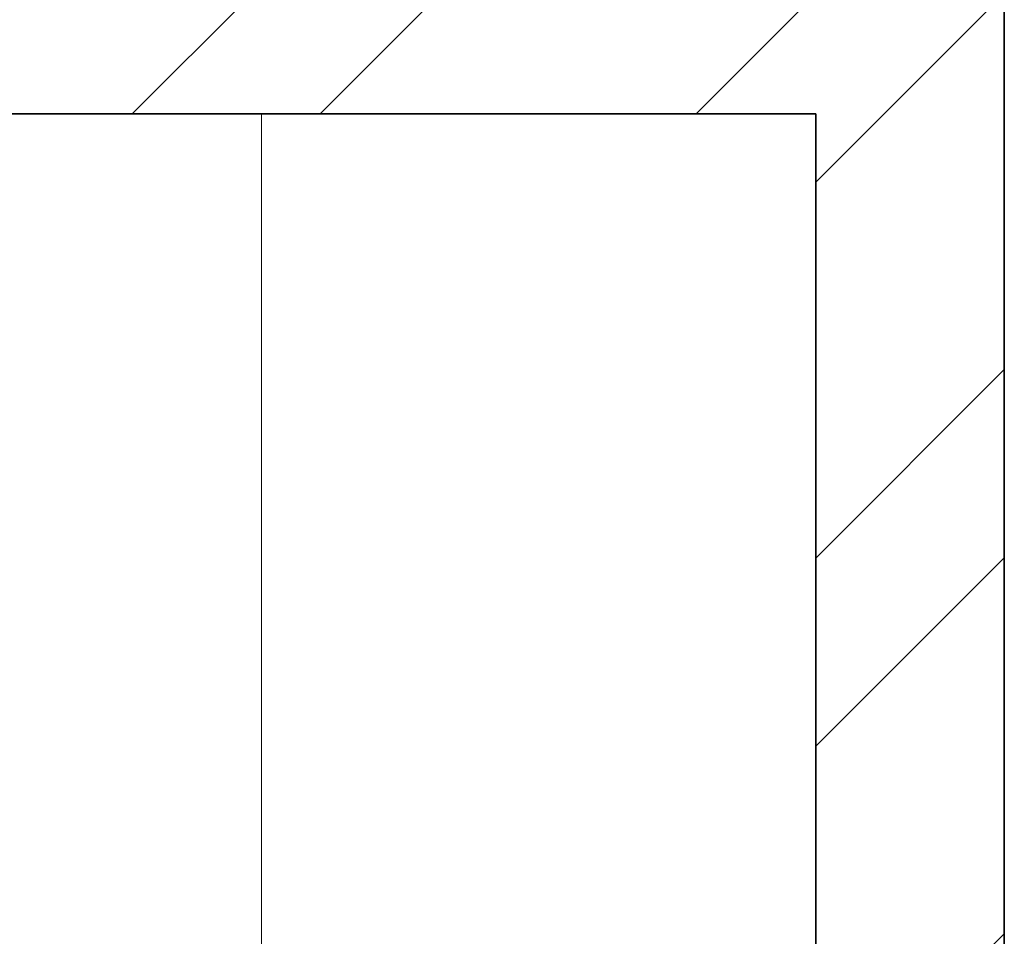
# Model space of a CAD drawing. Units: inches. Extents: x 1885 to 2748, y 783 to 2421.
# Tile 115 of 117: x 2595 to 2618, y 2093 to 2115. Entities that reach past the tile are written whole.
import ezdxf

# ---------------------------------------------------------------- set-up
doc = ezdxf.new("R2010")
doc.units = ezdxf.units.IN
doc.layers.add('A-FLOR-CASE', color=9, linetype='Continuous', lineweight=18)
doc.layers.add('A-WALL', color=7, linetype='Continuous', lineweight=35)
doc.layers.add('A-WALL-PATT', color=85, linetype='Continuous', lineweight=13, true_color=0x58ba48)

msp = doc.modelspace()

# ---------------------------------------------------------------- hatches: boundary and pattern name
at = {"layer": 'A-WALL-PATT'}
h = msp.add_hatch(dxfattribs=at)
h.set_pattern_fill('ANSI32', color=256)
h.paths.add_polyline_path([(2007.772, 2318.006), (1980.774, 2318.006), (1980.774, 2281.215), (1985.274, 2281.215), (1985.274, 2313.506), (2007.772, 2313.506), (2007.772, 2315.756)])
h.paths.add_polyline_path([(2094.324, 2318.006), (2067.772, 2318.006), (2067.772, 2313.506), (2094.324, 2313.506), (2094.324, 2315.756)])
h.paths.add_polyline_path([(2131.367, 2315.756), (2131.367, 2318.006), (2131.189, 2318.006), (2112.609, 2318.006), (2112.609, 2313.506), (2117.274, 2313.506), (2117.274, 2255.201), (2121.774, 2255.201), (2121.774, 2313.506), (2131.367, 2313.506)])
h.paths.add_polyline_path([(2190.512, 2318.006), (2155.367, 2318.006), (2155.367, 2313.506), (2169.774, 2313.506), (2169.774, 2229.506), (2121.774, 2229.506), (2121.774, 2233.451), (2119.524, 2233.451), (2117.274, 2233.451), (2117.274, 2201.101), (2121.774, 2201.101), (2121.774, 2225.006), (2169.774, 2225.006), (2169.774, 2165.006), (2306.274, 2165.006), (2306.274, 2066.006), (2310.774, 2066.006), (2344.274, 2066.006), (2486.274, 2066.006), (2486.274, 1886.006), (2483.02, 1886.006), (2483.02, 1881.506), (2486.274, 1881.506), (2486.274, 1880.678), (2490.774, 1880.678), (2490.774, 2070.506), (2344.274, 2070.506), (2310.774, 2070.506), (2310.774, 2165.006), (2310.774, 2173.636), (2308.524, 2173.636), (2306.274, 2173.636), (2306.274, 2169.506), (2174.274, 2169.506), (2174.274, 2313.506), (2190.512, 2313.506), (2190.512, 2315.756)])
h.paths.add_polyline_path([(1985.274, 2221.215), (1980.774, 2221.215), (1980.774, 2165.006), (1992.774, 2165.006), (1992.774, 2141.927), (1997.274, 2141.927), (1997.274, 2165.006), (2117.274, 2165.006), (2117.274, 2163.126), (2121.774, 2163.126), (2121.774, 2172.734), (2119.524, 2172.734), (2117.274, 2172.734), (2117.274, 2169.506), (1985.274, 2169.506)])
h.paths.add_polyline_path([(1997.274, 2105.927), (1992.774, 2105.927), (1992.774, 2070.506), (2016.774, 2070.506), (2016.774, 2059.123), (2019.024, 2059.123), (2021.274, 2059.123), (2021.274, 2070.506), (2117.274, 2070.506), (2117.274, 2022.506), (2114.423, 2022.506), (2114.423, 2018.006), (2123.627, 2018.006), (2123.627, 2020.256), (2123.627, 2022.506), (2121.774, 2022.506), (2121.774, 2142.587), (2119.524, 2142.587), (2117.274, 2142.587), (2117.274, 2075.006), (1997.274, 2075.006)])
h.paths.add_polyline_path([(2092.029, 2020.256), (2092.029, 2022.506), (2021.274, 2022.506), (2021.274, 2035.123), (2016.774, 2035.123), (2016.774, 2018.006), (2016.774, 1978.784), (2021.274, 1978.784), (2021.274, 2018.006), (2092.029, 2018.006)])
h.paths.add_polyline_path([(2260.938, 2022.506), (2153.105, 2022.506), (2153.105, 2020.256), (2153.105, 2018.006), (2155.274, 2018.006), (2155.274, 1886.006), (2107.629, 1886.006), (2107.629, 1881.506), (2182.911, 1881.506), (2182.911, 1883.756), (2182.911, 1886.006), (2159.774, 1886.006), (2159.774, 2018.006), (2260.938, 2018.006), (2260.938, 2020.256)])
h.paths.add_polyline_path([(2047.629, 1883.756), (2047.629, 1886.006), (2021.274, 1886.006), (2021.274, 1918.784), (2019.024, 1918.784), (2016.774, 1918.784), (2016.774, 1881.506), (2047.629, 1881.506)])
h.paths.add_polyline_path([(2306.361, 1883.756), (2306.361, 1886.006), (2296.274, 1886.006), (2296.274, 1982.006), (2316.535, 1982.006), (2316.535, 1984.256), (2316.535, 1986.506), (2296.274, 1986.506), (2296.274, 2022.506), (2289.276, 2022.506), (2289.276, 2018.006), (2291.774, 2018.006), (2291.774, 1886.006), (2242.911, 1886.006), (2242.911, 1881.506), (2306.361, 1881.506)], flags=17)
h.paths.add_polyline_path([(1985.274, 1843.006), (2021.6, 1843.006), (2021.534, 1845.441), (2021.477, 1847.506), (1980.774, 1847.506), (1980.774, 1809.446), (1985.274, 1809.446)])
h.paths.add_polyline_path([(2131.482, 1845.256), (2131.482, 1847.506), (2081.534, 1847.506), (2081.534, 1843.006), (2117.274, 1843.006), (2117.274, 1784.147), (2119.524, 1784.147), (2121.774, 1784.147), (2121.774, 1843.006), (2131.482, 1843.006)])
h.paths.add_polyline_path([(2203.886, 1847.506), (2155.482, 1847.506), (2155.482, 1843.006), (2169.774, 1843.006), (2169.774, 1759.006), (2121.774, 1759.006), (2121.774, 1761.457), (2117.274, 1761.457), (2117.274, 1730.429), (2121.774, 1730.429), (2121.774, 1754.506), (2177.421, 1754.506), (2177.421, 1756.756), (2177.421, 1759.006), (2174.274, 1759.006), (2174.274, 1843.006), (2203.886, 1843.006)])
h.paths.add_polyline_path([(2335.554, 1845.256), (2335.554, 1847.506), (2239.886, 1847.506), (2239.886, 1843.006), (2306.274, 1843.006), (2306.274, 1759.006), (2199.486, 1759.006), (2199.486, 1754.506), (2310.774, 1754.506), (2310.774, 1843.006), (2335.554, 1843.006)])
h.paths.add_polyline_path([(2348.774, 2022.506), (2344.274, 2022.506), (2344.274, 1986.506), (2341.681, 1986.506), (2341.681, 1982.006), (2344.274, 1982.006), (2344.274, 1886.006), (2330.361, 1886.006), (2330.361, 1881.506), (2361.627, 1881.506), (2361.627, 1883.756), (2361.627, 1886.006), (2348.774, 1886.006)], flags=17)
h.paths.add_polyline_path([(2283.251, 2315.756), (2283.251, 2318.006), (2238.512, 2318.006), (2238.512, 2313.506), (2283.251, 2313.506)], flags=17)
h.paths.add_polyline_path([(2363.274, 2348.006), (2388.677, 2348.006), (2388.677, 2350.256), (2388.677, 2352.506), (2358.774, 2352.506), (2358.774, 2348.006), (2358.774, 2318.006), (2344.481, 2318.006), (2344.481, 2313.506), (2358.774, 2313.506), (2358.774, 2229.506), (2310.774, 2229.506), (2310.774, 2231.952), (2306.274, 2231.952), (2306.274, 2205.611), (2310.774, 2205.611), (2310.774, 2225.006), (2358.774, 2225.006), (2358.774, 2211.506), (2452.329, 2211.506), (2452.329, 2213.756), (2452.329, 2216.006), (2363.274, 2216.006), (2363.274, 2318.006)])
h.paths.add_polyline_path([(2310.774, 2313.506), (2320.481, 2313.506), (2320.481, 2315.756), (2320.481, 2318.006), (2302.728, 2318.006), (2302.728, 2313.506), (2306.274, 2313.506), (2306.274, 2251.076), (2310.774, 2251.076)], flags=17)
h.paths.add_polyline_path([(2490.774, 2352.506), (2486.274, 2352.506), (2448.677, 2352.506), (2448.677, 2348.006), (2486.274, 2348.006), (2486.274, 2318.006), (2486.274, 2216.006), (2481.78, 2216.006), (2481.78, 2211.506), (2486.274, 2211.506), (2486.274, 2165.006), (2493.289, 2165.006), (2493.289, 2167.256), (2493.289, 2169.506), (2490.774, 2169.506), (2490.774, 2313.506), (2494.429, 2313.506), (2494.429, 2318.006), (2490.774, 2318.006)])
h.paths.add_polyline_path([(2534.653, 2318.006), (2515.691, 2318.006), (2515.691, 2313.506), (2534.653, 2313.506), (2534.653, 2315.756)])
h.paths.add_polyline_path([(2618.274, 2318.006), (2594.653, 2318.006), (2594.653, 2313.506), (2613.774, 2313.506), (2613.774, 2281.706), (2618.274, 2281.706)])
h.paths.add_polyline_path([(2618.274, 2221.706), (2613.774, 2221.706), (2613.774, 2169.506), (2554.019, 2169.506), (2554.019, 2165.006), (2613.774, 2165.006), (2613.774, 2152.878), (2618.274, 2152.878)])
h.paths.add_polyline_path([(2618.274, 2128.878), (2616.024, 2128.878), (2613.774, 2128.878), (2613.774, 2117.006), (2529.774, 2117.006), (2529.774, 2165.006), (2532.848, 2165.006), (2532.848, 2169.506), (2522.867, 2169.506), (2522.867, 2165.006), (2525.274, 2165.006), (2525.274, 2117.006), (2525.274, 2112.506), (2525.274, 2108.576), (2529.774, 2108.576), (2529.774, 2112.506), (2613.774, 2112.506), (2613.774, 2080.19), (2618.274, 2080.19)])
h.paths.add_polyline_path([(2618.274, 2044.19), (2616.024, 2044.19), (2613.774, 2044.19), (2613.774, 2015.506), (2529.774, 2015.506), (2529.774, 2088.582), (2527.524, 2088.582), (2525.274, 2088.582), (2525.274, 2011.006), (2613.774, 2011.006), (2613.774, 1956.755), (2618.274, 1956.755)])
h.paths.add_polyline_path([(2618.274, 1881.506), (2618.274, 1896.755), (2613.774, 1896.755), (2613.774, 1881.506), (2613.774, 1847.506), (2592.715, 1847.506), (2592.715, 1843.006), (2613.774, 1843.006), (2613.774, 1765.006), (2613.774, 1760.506), (2609.621, 1760.506), (2609.621, 1756.006), (2613.774, 1756.006), (2613.774, 1660.006), (2608.544, 1660.006), (2608.544, 1655.506), (2613.774, 1655.506), (2613.774, 1508.158), (2618.274, 1508.158)])
h.paths.add_polyline_path([(2565.774, 1843.006), (2568.997, 1843.006), (2568.997, 1847.506), (2490.774, 1847.506), (2490.774, 1849.7), (2488.524, 1849.7), (2486.274, 1849.7), (2486.274, 1847.506), (2477.274, 1847.506), (2477.274, 1838.506), (2477.274, 1821.493), (2486.274, 1821.493), (2486.274, 1838.506), (2561.274, 1838.506), (2561.274, 1765.006), (2486.274, 1765.006), (2486.274, 1786.157), (2477.274, 1786.157), (2477.274, 1765.006), (2477.274, 1756.006), (2486.274, 1756.006), (2565.774, 1756.006), (2585.621, 1756.006), (2585.621, 1758.256), (2585.621, 1760.506), (2565.774, 1760.506), (2565.774, 1765.006)])
h.paths.add_polyline_path([(2486.274, 1651.006), (2561.274, 1651.006), (2561.274, 1567.006), (2486.274, 1567.006), (2486.274, 1591.321), (2477.274, 1591.321), (2477.274, 1567.006), (2477.274, 1558.006), (2477.274, 1555.439), (2481.774, 1555.439), (2481.774, 1558.006), (2568.653, 1558.006), (2568.653, 1560.256), (2568.653, 1562.506), (2565.774, 1562.506), (2565.774, 1655.506), (2584.544, 1655.506), (2584.544, 1657.756), (2584.544, 1660.006), (2565.774, 1660.006), (2486.274, 1660.006), (2477.274, 1660.006), (2477.274, 1651.006), (2477.274, 1632.989), (2486.274, 1632.989)])
h.paths.add_polyline_path([(2449.967, 1883.756), (2449.967, 1886.006), (2421.627, 1886.006), (2421.627, 1881.506), (2449.967, 1881.506)], flags=17)
h.paths.add_polyline_path([(2447.274, 1847.506), (2395.554, 1847.506), (2395.554, 1843.006), (2442.774, 1843.006), (2442.774, 1809.27), (2447.274, 1809.27)])
h.paths.add_polyline_path([(1985.274, 1749.446), (1980.774, 1749.446), (1980.774, 1694.504), (1985.274, 1694.504), (1985.274, 1694.506), (1986.897, 1694.506), (1986.897, 1697.78), (1986.897, 1699.006), (1985.274, 1699.006)])
h.paths.add_polyline_path([(2152.774, 1699.006), (2121.774, 1699.006), (2121.774, 1703.668), (2119.524, 1703.668), (2117.274, 1703.668), (2117.274, 1699.006), (2009.219, 1699.006), (2009.219, 1694.506), (2148.274, 1694.506), (2148.274, 1692.631), (2152.774, 1692.631)])
h.paths.add_polyline_path([(2016.274, 1694.506), (2011.774, 1694.506), (2011.774, 1558.006), (2040.806, 1558.006), (2040.806, 1560.256), (2040.806, 1562.506), (2016.274, 1562.506)])
h.paths.add_polyline_path([(2152.774, 1663.017), (2150.524, 1663.017), (2148.274, 1663.017), (2148.274, 1562.506), (2100.806, 1562.506), (2100.806, 1558.006), (2165.119, 1558.006), (2165.119, 1560.256), (2165.119, 1562.506), (2152.774, 1562.506), (2152.774, 1610.506), (2224.774, 1610.506), (2224.774, 1607.99), (2229.274, 1607.99), (2229.274, 1615.006), (2152.774, 1615.006)])
h.paths.add_polyline_path([(2238.613, 1560.256), (2238.613, 1562.506), (2229.274, 1562.506), (2229.274, 1588.756), (2227.024, 1588.763), (2224.774, 1588.771), (2224.774, 1562.506), (2189.119, 1562.506), (2189.119, 1558.006), (2238.613, 1558.006)])
h.paths.add_polyline_path([(2336.024, 1560.256), (2336.024, 1562.506), (2310.774, 1562.506), (2310.774, 1656.347), (2308.524, 1656.347), (2306.274, 1656.347), (2306.274, 1562.506), (2286.613, 1562.506), (2286.613, 1558.006), (2336.024, 1558.006)])
h.paths.add_polyline_path([(2447.274, 1690.968), (2445.024, 1690.968), (2442.774, 1690.968), (2442.774, 1687.006), (2306.274, 1687.006), (2306.274, 1680.75), (2310.774, 1680.75), (2310.774, 1682.506), (2442.774, 1682.506), (2442.774, 1562.506), (2396.024, 1562.506), (2396.024, 1558.006), (2447.274, 1558.006)])
h.paths.add_polyline_path([(2447.274, 1749.27), (2445.024, 1749.27), (2442.774, 1749.27), (2442.774, 1717.232), (2447.274, 1717.232)])
h.paths.add_polyline_path([(2044.674, 1521.756), (2044.674, 1524.006), (2007.274, 1524.006), (2007.274, 1503.49), (2009.524, 1503.49), (2011.774, 1503.49), (2011.774, 1519.506), (2044.674, 1519.506)])
h.paths.add_polyline_path([(2177.969, 1521.756), (2177.969, 1524.006), (2104.674, 1524.006), (2104.674, 1519.506), (2145.774, 1519.506), (2145.774, 1387.506), (2143.37, 1387.506), (2143.37, 1383.006), (2251.585, 1383.006), (2251.585, 1385.256), (2251.585, 1387.506), (2150.274, 1387.506), (2150.274, 1519.506), (2177.969, 1519.506)])
h.paths.add_polyline_path([(2298.704, 1524.006), (2237.969, 1524.006), (2237.969, 1519.506), (2282.274, 1519.506), (2282.274, 1387.506), (2279.683, 1387.506), (2279.683, 1383.006), (2286.774, 1383.006), (2286.774, 1419.006), (2312.451, 1419.006), (2312.451, 1421.256), (2312.451, 1423.506), (2286.774, 1423.506), (2286.774, 1519.506), (2298.704, 1519.506), (2298.704, 1521.722)], flags=17)
h.paths.add_polyline_path([(2361.897, 1521.756), (2361.897, 1524.006), (2322.704, 1524.006), (2322.704, 1519.506), (2334.774, 1519.506), (2334.774, 1423.506), (2331.93, 1423.506), (2331.93, 1419.006), (2334.774, 1419.006), (2334.774, 1387.506), (2334.774, 1383.228), (2339.274, 1383.228), (2339.274, 1387.506), (2339.274, 1519.506), (2361.897, 1519.506)], flags=17)
h.paths.add_polyline_path([(2447.274, 1521.756), (2447.274, 1524.006), (2421.897, 1524.006), (2421.897, 1519.506), (2447.274, 1519.506)], flags=17)
h.paths.add_polyline_path([(2481.774, 1529.6), (2479.524, 1529.6), (2477.274, 1529.6), (2477.274, 1524.006), (2474.489, 1524.006), (2474.489, 1519.506), (2477.274, 1519.506), (2477.274, 1334.506), (2296.774, 1334.506), (2296.774, 1240.506), (2160.274, 1240.506), (2160.274, 1180.506), (2112.274, 1180.506), (2112.274, 1207.692), (2110.024, 1207.692), (2107.774, 1207.692), (2107.774, 1171.609), (2112.274, 1171.609), (2112.274, 1176.006), (2160.274, 1176.006), (2160.274, 1092.006), (2144.221, 1092.006), (2144.221, 1087.506), (2189.497, 1087.506), (2189.497, 1089.756), (2189.497, 1092.006), (2164.774, 1092.006), (2164.774, 1236.006), (2296.774, 1236.006), (2296.774, 1231.912), (2301.274, 1231.912), (2301.274, 1330.006), (2481.774, 1330.006), (2481.774, 1387.506)])
h.paths.add_polyline_path([(2618.274, 1448.158), (2613.774, 1448.158), (2613.774, 1382.506), (2529.774, 1382.506), (2525.274, 1382.506), (2525.274, 1307.062), (2529.774, 1307.062), (2529.774, 1378.006), (2613.774, 1378.006), (2613.774, 1354.988), (2618.274, 1354.988)])
h.paths.add_polyline_path([(2618.274, 1318.988), (2613.774, 1318.988), (2613.774, 1281.006), (2529.774, 1281.006), (2529.774, 1283.786), (2527.524, 1283.786), (2525.274, 1283.786), (2525.274, 1228.506), (2516.794, 1228.506), (2516.794, 1224.006), (2533.484, 1224.006), (2533.484, 1226.256), (2533.484, 1228.506), (2529.774, 1228.506), (2529.774, 1276.506), (2613.774, 1276.506), (2613.774, 1266.02), (2618.274, 1266.02)])
h.paths.add_polyline_path([(2618.274, 1134.964), (2613.774, 1134.964), (2613.774, 1092.006), (2594.545, 1092.006), (2594.545, 1087.506), (2618.274, 1087.506)])
h.paths.add_polyline_path([(2534.545, 1092.006), (2509.765, 1092.006), (2509.765, 1087.506), (2534.545, 1087.506), (2534.545, 1089.756)])
h.paths.add_polyline_path([(2481.274, 1224.006), (2484.117, 1224.006), (2484.117, 1226.256), (2484.117, 1228.506), (2476.774, 1228.506), (2476.774, 1198.506), (2471.61, 1198.506), (2471.61, 1194.006), (2476.774, 1194.006), (2476.774, 1062.006), (2436.894, 1062.006), (2436.894, 1057.506), (2476.774, 1057.506), (2481.274, 1057.506), (2481.274, 1062.006), (2481.274, 1087.506), (2485.354, 1087.506), (2485.354, 1089.756), (2485.354, 1092.006), (2481.274, 1092.006), (2481.274, 1117.506)])
h.paths.add_polyline_path([(2439.898, 1198.506), (2349.274, 1198.506), (2349.274, 1194.006), (2349.274, 1180.506), (2301.274, 1180.506), (2301.274, 1201.896), (2299.024, 1201.896), (2296.774, 1201.896), (2296.774, 1172.335), (2299.024, 1172.335), (2301.274, 1172.335), (2301.274, 1176.006), (2349.274, 1176.006), (2349.274, 1092.006), (2334.452, 1092.006), (2334.452, 1087.506), (2349.274, 1087.506), (2349.274, 1057.506), (2353.774, 1057.506), (2376.894, 1057.506), (2376.894, 1059.756), (2376.894, 1062.006), (2353.774, 1062.006), (2353.774, 1087.506), (2353.774, 1180.506), (2353.774, 1194.006), (2439.898, 1194.006), (2439.898, 1196.256)])
h.paths.add_polyline_path([(2270.596, 1089.756), (2270.596, 1092.006), (2249.497, 1092.006), (2249.497, 1087.506), (2270.596, 1087.506)], flags=17)
h.paths.add_polyline_path([(2310.452, 1092.006), (2301.274, 1092.006), (2301.274, 1153.292), (2296.774, 1153.292), (2296.774, 1092.006), (2293.786, 1092.006), (2293.786, 1087.506), (2310.452, 1087.506), (2310.452, 1089.756)], flags=17)
h.paths.add_polyline_path([(2112.274, 1150.328), (2110.024, 1150.328), (2107.774, 1150.328), (2107.774, 1092.006), (2104.465, 1092.006), (2104.465, 1087.506), (2120.221, 1087.506), (2120.221, 1089.756), (2120.221, 1092.006), (2112.274, 1092.006)])
h.paths.add_polyline_path([(2082.172, 1092.006), (2058.144, 1092.006), (2058.144, 1087.506), (2082.172, 1087.506), (2082.172, 1089.756)])
h.paths.add_polyline_path([(1975.774, 1145.638), (1971.274, 1145.638), (1971.274, 1087.506), (1980.774, 1087.506), (1998.144, 1087.506), (1998.144, 1089.756), (1998.144, 1092.006), (1985.274, 1092.006), (1975.774, 1092.006)])
h.paths.add_polyline_path([(2112.274, 1244.385), (2110.024, 1244.385), (2107.774, 1244.385), (2107.774, 1240.506), (1992.274, 1240.506), (1992.274, 1271.008), (1987.774, 1271.008), (1987.774, 1240.506), (1980.774, 1240.506), (1975.774, 1240.506), (1971.274, 1240.506), (1971.274, 1205.638), (1975.774, 1205.638), (1975.774, 1236.006), (2107.774, 1236.006), (2107.774, 1233.444), (2112.274, 1233.444), (2112.274, 1236.006)])
h.paths.add_polyline_path([(2112.274, 1383.006), (2114.783, 1383.006), (2114.783, 1385.256), (2114.783, 1387.506), (2102.476, 1387.506), (2102.476, 1383.006), (2107.774, 1383.006), (2107.774, 1335.006), (2011.774, 1335.006), (2011.774, 1349.939), (2007.274, 1349.939), (2007.274, 1335.006), (1987.774, 1335.006), (1987.774, 1330.506), (1987.774, 1307.008), (1992.274, 1307.008), (1992.274, 1330.506), (2007.274, 1330.506), (2107.774, 1330.506), (2107.774, 1264.711), (2112.274, 1264.711)])
h.paths.add_polyline_path([(2077.857, 1387.506), (2011.774, 1387.506), (2011.774, 1390.036), (2009.524, 1390.036), (2007.274, 1390.036), (2007.274, 1373.939), (2011.774, 1373.939), (2011.774, 1383.006), (2077.857, 1383.006)])
h.paths.add_polyline_path([(2011.774, 1443.49), (2007.274, 1443.49), (2007.274, 1410.248), (2011.774, 1410.248)])

# ---------------------------------------------------------------- linework, layer by layer
at = {"layer": 'A-FLOR-CASE'}
msp.add_line((2600.531, 2112.506), (2600.531, 2028.584), dxfattribs=at)
at = {"layer": 'A-WALL'}
for p, q in [((2618.274, 2128.878), (2618.274, 2080.19)), ((2529.774, 2112.506), (2613.774, 2112.506)), ((2613.774, 2112.506), (2613.774, 2080.19))]:
    msp.add_line(p, q, dxfattribs=at)

doc.saveas('drawing.dxf')
